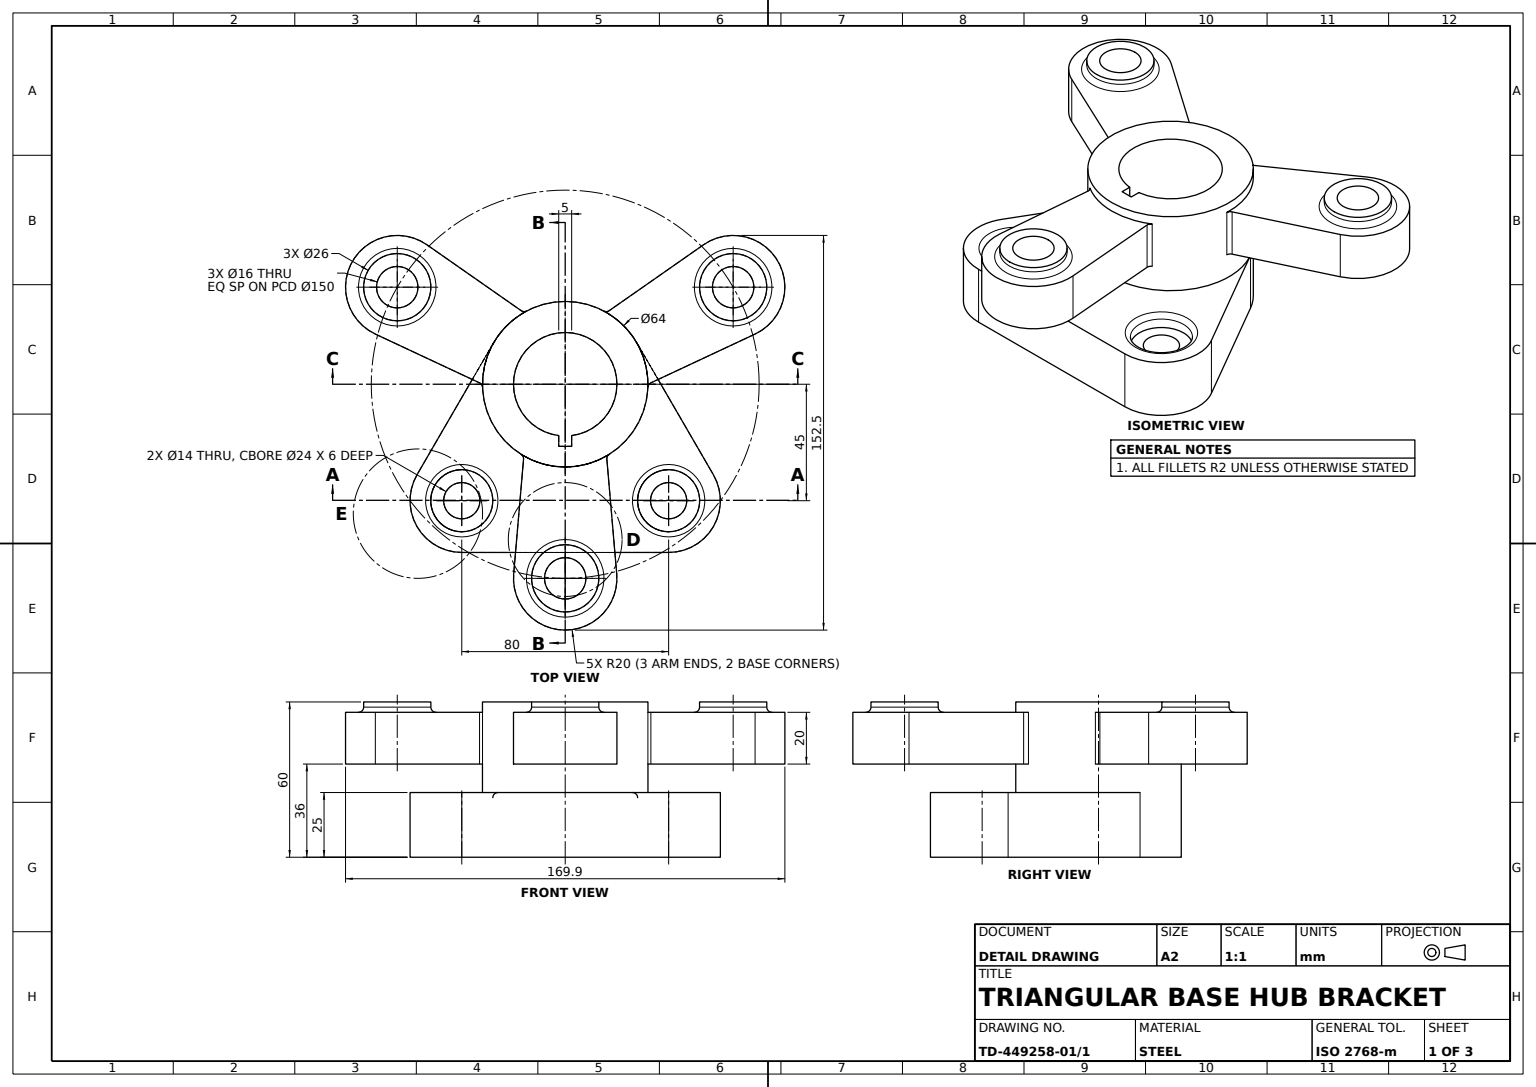
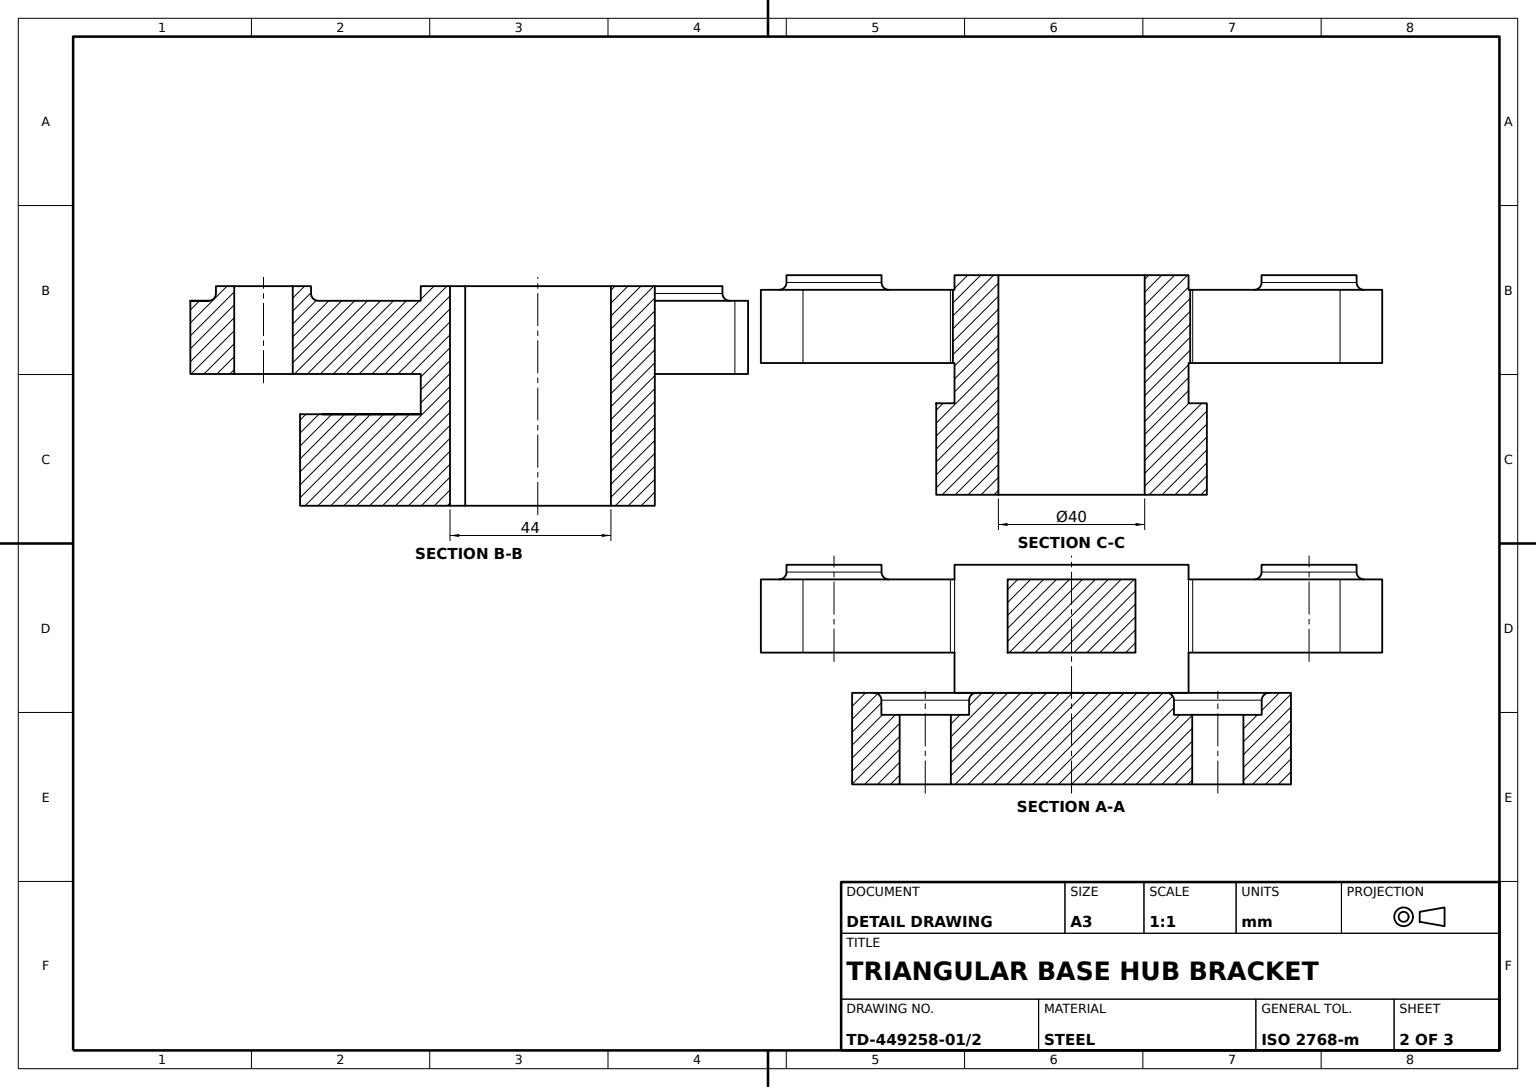
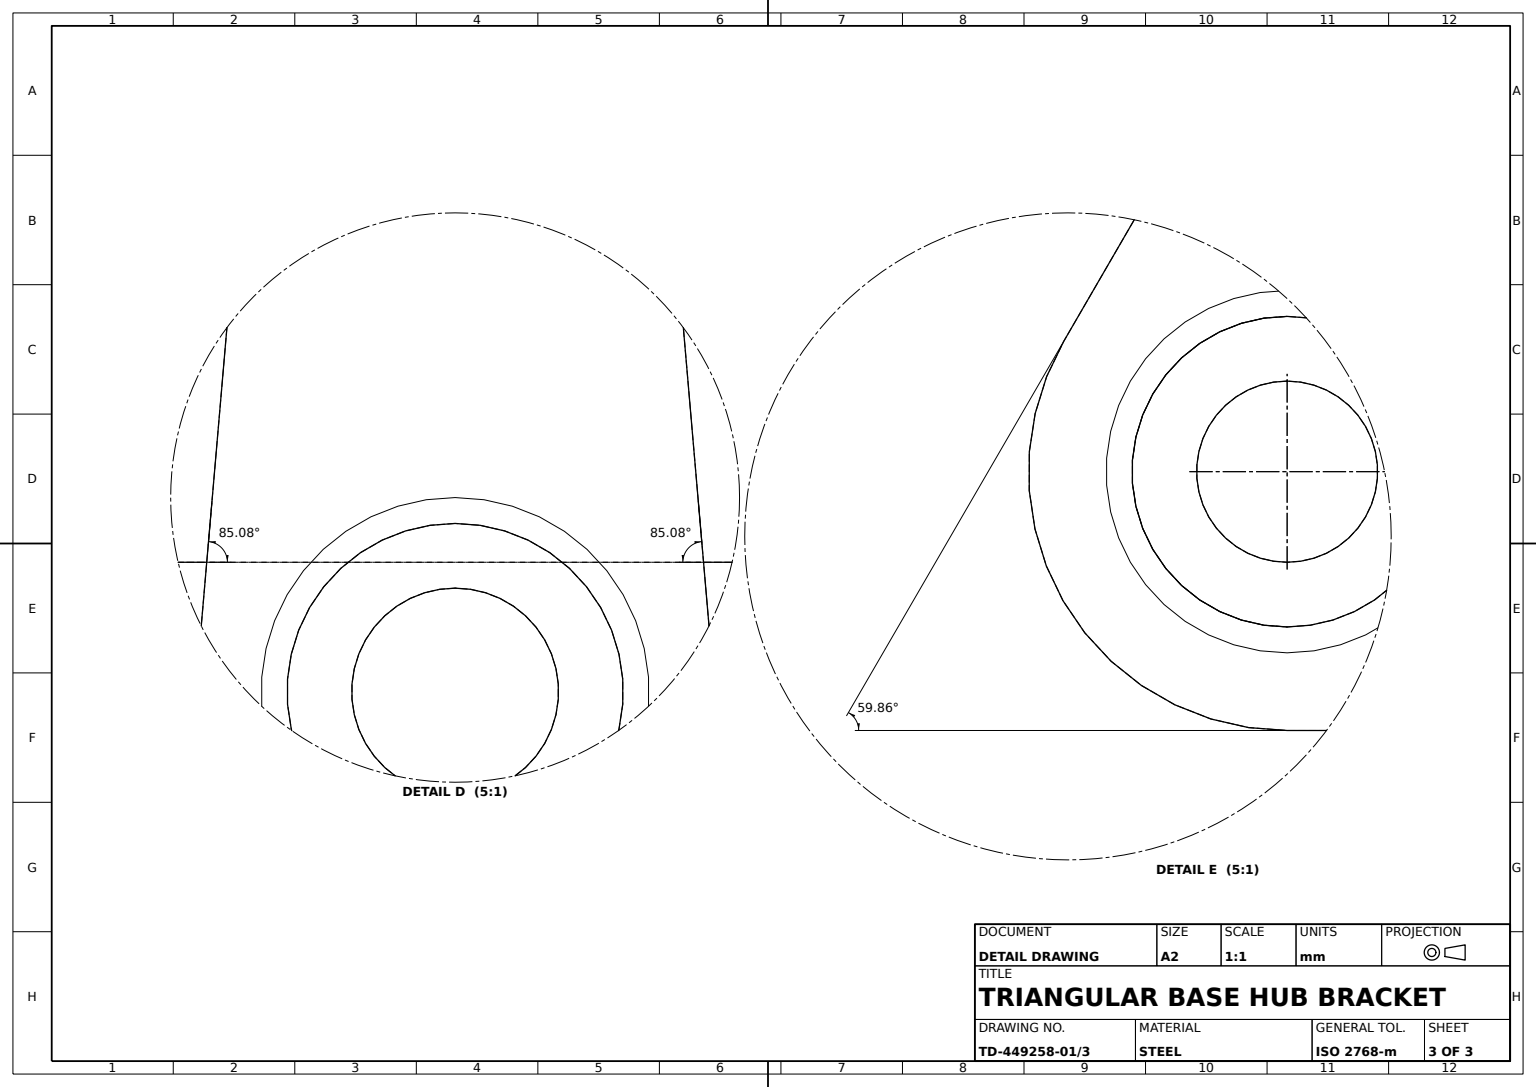
from build123d import *

# Parameters (mm, degrees)
BASE_PLATE_DEPTH                  = 25
SKETCH1_15_R                      = 32
HUB_DEPTH                         = 60
KEYWAY_CUT_DEPTH                  = 96.131487952
COUNTERBORED_HOLES_M8_D           = 14
COUNTERBORED_HOLES_M8_CBORE_D     = 24
COUNTERBORED_HOLES_M8_CBORE_DEPTH = 6
ARM_START                         = -24
ARM_SKETCH_R                      = 8
ARM_DEPTH                         = 20
SKETCH7_3_R                       = 13
SKETCH7_3_R_2                     = 8
ARM_END_BOSS_DEPTH                = 24
ARM_PATTERN_3X_COUNT              = 3
ARM_FILLETS_R2_R                  = 2
COUNTERBORE_EDGE_FILLETS_R2_R     = 2


with BuildPart() as part:
    # Base and Hub Sketch → Base Plate (new body)
    with BuildSketch(Plane(origin=(0, 0, 0), x_dir=(1, 0, 0), z_dir=(0, 1, 0))):
        with BuildLine():
            Line((-40, -65), (40, -65))
            ThreePointArc((40, -65), (57.332449137, -54.979288897), (57.296551724, -34.95862069))
            Line((57.296551724, -34.95862069), (27.674482759, 16.066206897))
            ThreePointArc((27.674482759, 16.066206897), (0, 32), (-27.674482759, 16.066206897))
            Line((-27.674482759, 16.066206897), (-57.296551724, -34.95862069))
            ThreePointArc((-57.296551724, -34.95862069), (-57.332449137, -54.979288897), (-40, -65))
        make_face()
    extrude(amount=BASE_PLATE_DEPTH)

    # Sketch1_15 → Hub (add)
    with BuildSketch(Plane(origin=(0, 0, 0), x_dir=(1, 0, 0), z_dir=(0, 1, 0))):
        with Locations(Location((0, 0, 0), (0, 0, 149.863023681))):
            Circle(SKETCH1_15_R)
        with BuildLine():
            Line((2.5, -19.843134833), (2.5, -24))
            Line((2.5, -24), (-2.5, -24))
            Line((-2.5, -24), (-2.5, -19.843134833))
            ThreePointArc((-2.5, -19.843134833), (0, 20), (2.5, -19.843134833))
        make_face(mode=Mode.SUBTRACT)
    extrude(amount=HUB_DEPTH)

    # Keyway Sketch → Keyway Cut (cut, through all)
    with BuildSketch(Plane(origin=(0, 25, 0), x_dir=(1, 0, 0), z_dir=(0, 1, 0))):
        with BuildLine():
            Line((-2.5, -24), (2.5, -24))
            Line((2.5, -24), (2.5, -19.843134833))
            ThreePointArc((2.5, -19.843134833), (0, 20), (-2.5, -19.843134833))
            Line((-2.5, -19.843134833), (-2.5, -24))
        make_face()
    extrude(amount=-KEYWAY_CUT_DEPTH, mode=Mode.SUBTRACT)

    # Counterbored Holes M8 (through all)
    with Locations(Plane(origin=(0, 25, 0), x_dir=(1, 0, 0), z_dir=(0, 1, 0))):
        with Locations((-40, -45), (40, -45)):
            CounterBoreHole(COUNTERBORED_HOLES_M8_D / 2, COUNTERBORED_HOLES_M8_CBORE_D / 2, COUNTERBORED_HOLES_M8_CBORE_DEPTH)

    # Arm Sketch → Arm (add)
    with BuildSketch(Plane(origin=(0, 60, 0), x_dir=(1, 0, 0), z_dir=(0, 1, 0)).offset(ARM_START)):
        with BuildLine():
            Line((53.502050444, 53.898195759), (16, 27.712812921))
            ThreePointArc((16, 27.712812921), (27.712812921, 16), (32, 0))
            Line((32, 0), (73.428231967, 19.385036959))
            ThreePointArc((73.428231967, 19.385036959), (82.27241336, 47.5), (53.502050444, 53.898195759))
        make_face()
        with Locations(Location((64.951905284, 37.5, 0), (0, 0, 270))):
            Circle(ARM_SKETCH_R, mode=Mode.SUBTRACT)
    arm = extrude(amount=ARM_DEPTH)

    # Sketch7_3 → Arm End Boss (add)
    with BuildSketch(Plane(origin=(0, 60, 0), x_dir=(1, 0, 0), z_dir=(0, 1, 0)).offset(ARM_START)):
        with Locations(Location((64.951905284, 37.5, 0), (0, 0, 270))):
            Circle(SKETCH7_3_R)
        with Locations(Location((64.951905284, 37.5, 0), (0, 0, 270))):
            Circle(SKETCH7_3_R_2, mode=Mode.SUBTRACT)
    arm_end_boss = extrude(amount=ARM_END_BOSS_DEPTH)

    # Arm Pattern 3x: Arm, Arm End Boss ×3 about axis
    arm_pattern_3x_axis = Axis((0, 0, 0), (0, 1, 0))
    add([arm.rotate(arm_pattern_3x_axis, i * 360 / ARM_PATTERN_3X_COUNT) for i in range(1, ARM_PATTERN_3X_COUNT)])
    add([arm_end_boss.rotate(arm_pattern_3x_axis, i * 360 / ARM_PATTERN_3X_COUNT) for i in range(1, ARM_PATTERN_3X_COUNT)])

    # Arm Fillets R2
    arm_fillets_r2_edges = [part.edges().sort_by_distance(p)[0] for p in [
        (64.951905284, 56, -50.5),
        (-16, 46, 27.712812921),
        (16, 46, 27.712812921),
        (-16, 46, -27.712812921),
        (-32, 46, 0),
        (11.258330249, 56, 81.5),
        (-76.210235533, 56, -31),
        (32, 46, 0),
        (16, 46, -27.712812921),
    ]]
    fillet(arm_fillets_r2_edges, radius=ARM_FILLETS_R2_R)

    # Counterbore Edge Fillets R2
    counterbore_edge_fillets_r2_edges = [part.edges().sort_by_distance(p)[0] for p in [
        (28, 25, 45),
        (-52, 25, 45),
    ]]
    fillet(counterbore_edge_fillets_r2_edges, radius=COUNTERBORE_EDGE_FILLETS_R2_R)


solid = part.part
